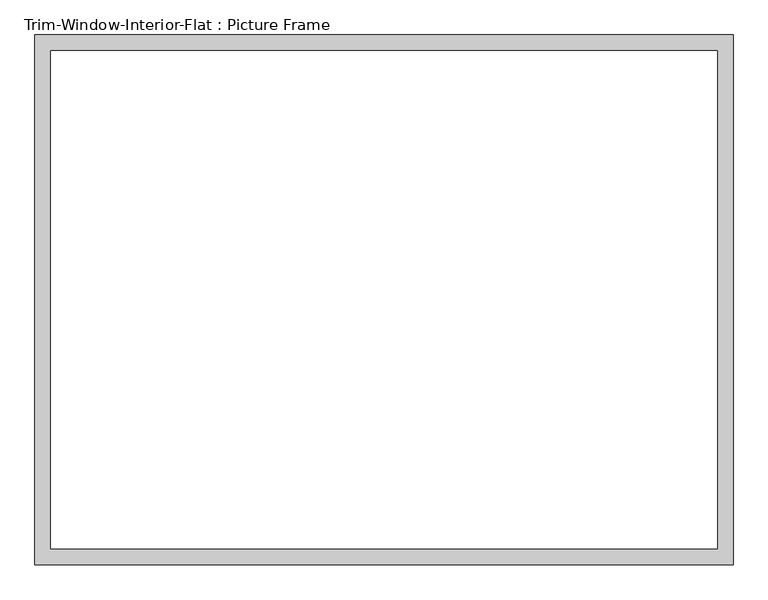
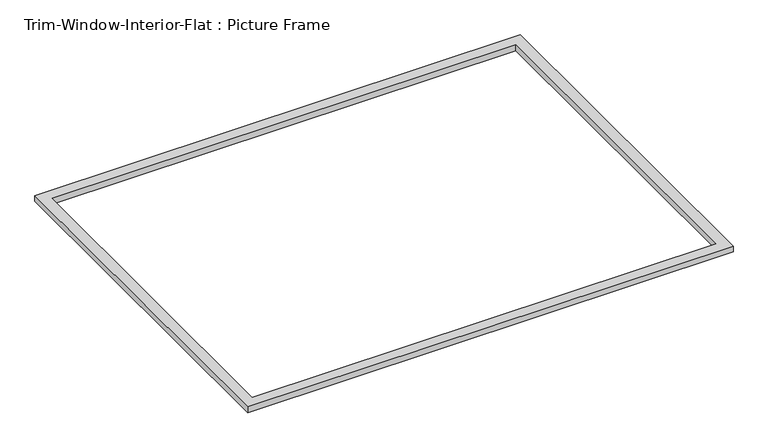
"""IFC4 building model written with IfcOpenShell, lengths in millimetres: proxy geometry, Trim-Window-Interior-Flat : Picture Frame."""

from ifc_helpers import new_model, si_unit, origin, origin_with_axes, place, context, project, spatial, polyline, outline, extrude, source, transform, mapped, element, save


def trim_window_interior_flat_picture_frame_939a8053(model_context):
    return source(origin(), model_context, "Body", "SweptSolid", [
        extrude(outline(polyline([(1263.65, 44.45), (1263.65, -1873.25), (-1263.65, -1873.25), (-1263.65, 44.45), (1263.65, 44.45)]), holes=[polyline([(1206.5, -12.7), (-1206.5, -12.7), (-1206.5, -1816.1), (1206.5, -1816.1), (1206.5, -12.7)])]), origin_with_axes(), (0.0, 0.0, 1.0), 31.75),
    ])


if __name__ == "__main__":
    model = new_model("IFC4")
    model_context = context("Model", 3, world=origin())
    ifc_project = project(units=[si_unit("LENGTHUNIT", "METRE", prefix="MILLI")], contexts=[model_context])
    site = spatial("IfcSite", under=ifc_project)
    building = spatial("IfcBuilding", under=site)
    placement = place(None, origin())
    trim_window_interior_flat_picture_frame_shape = trim_window_interior_flat_picture_frame_939a8053(model_context)
    element("IfcBuildingElementProxy", 1, Name="Trim-Window-Interior-Flat : Picture Frame", ObjectType="Trim-Window-Interior-Flat : Picture Frame", at=placement, inside=building, context=model_context, shape_type="MappedRepresentation", body=[
        mapped(trim_window_interior_flat_picture_frame_shape, transform((0.0, 0.0, 0.0), x_axis=(1.0, 0.0, 0.0), y_axis=(0.0, 1.0, 0.0), z_axis=(0.0, 0.0, 1.0))),
    ])
    save(model, "model.ifc")

# Revit data of these elements
# Type "Trim-Window-Interior-Flat : Picture Frame"
#   Trim Thickness_Picture Frame = 0' - 1 1/4"
#   Trim Width = 0' - 2 1/4"
#   Trim Thickness_with Sill = 0' - 0 3/4"
#   Sill Thickness = 0' - 1 1/4"
#   Opening Width [instance default] = 2' - 0"
#   Opening Height [instance default] = 3' - 0"
#   Default Elevation = 4' - 0"
#   Sill = no
#   Picture Frame = yes
#   Trim Material [instance default] = none
# Element 1 (IfcBuildingElementProxy, "Trim-Window-Interior-Flat : Picture Frame")
#   Opening Width = 8' - 0"
#   Opening Height = 6' - 0"
#   Trim Material = Wood - Stained
#   Materials on its faces: "Wood - Stained"
# Materials
#   "Wood - Stained": class "Wood", colour RGB 224 178 126, transparency 0, Cost = 0
